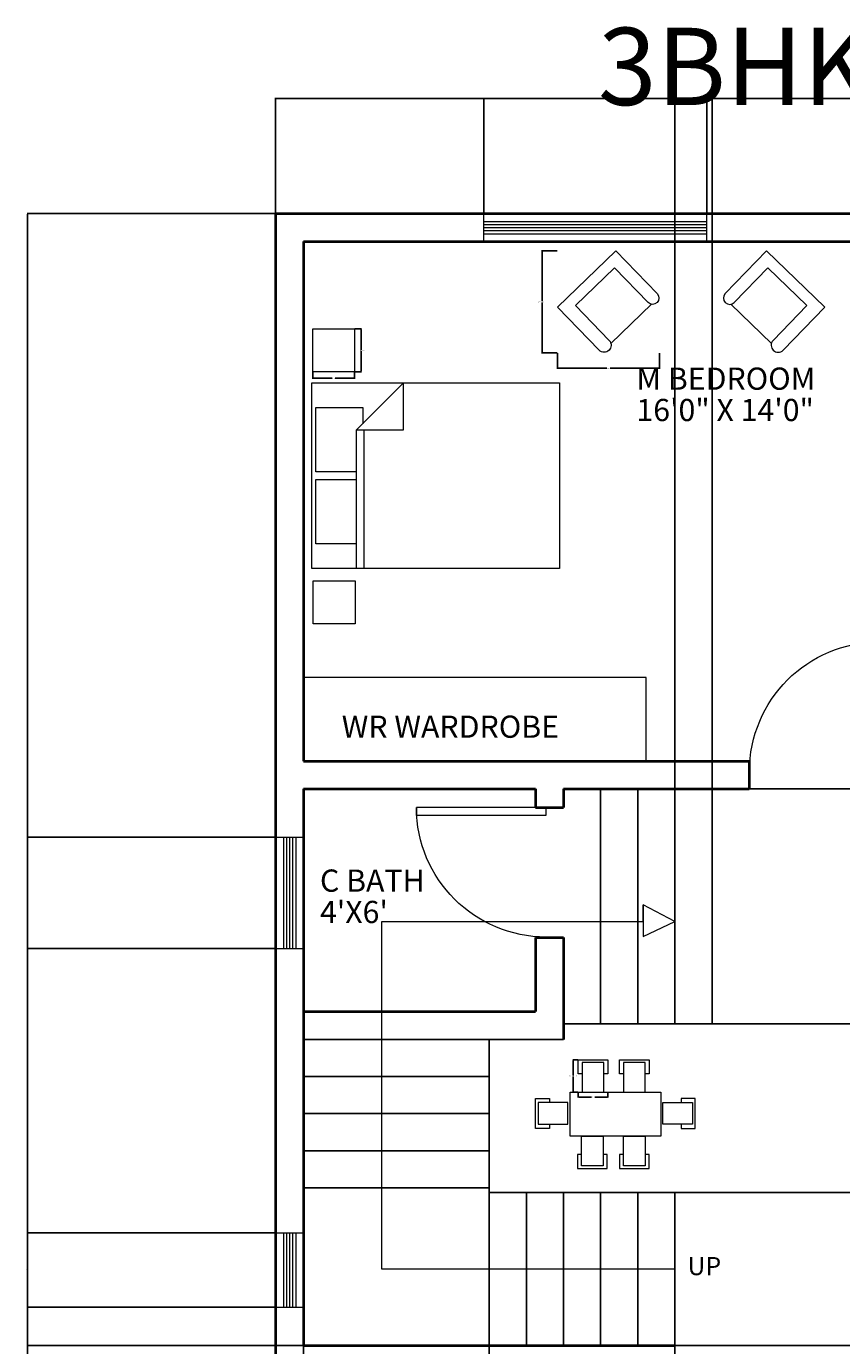
# Model space of a CAD drawing. Units: inches. Extents: x 12978 to 13669, y 46550 to 47327.
# Tile 3 of 5: x 12978 to 13242, y 46901 to 47327. Entities that reach past the tile are written whole.
import ezdxf

# ---------------------------------------------------------------- set-up
doc = ezdxf.new("R2010")
doc.units = ezdxf.units.IN
for name, color, linetype, lineweight in [('A-ANNO-DIMS', 2, 'Continuous', 18), ('A-ANNO-SYMB', 7, 'Continuous', 18), ('A-ANNO-TITL', 7, 'Continuous', 35), ('A-AREA-IDEN', 1, 'Continuous', 18), ('A-FLOR-CASE', 8, 'Continuous', 20), ('door', 4, 'Continuous', 20), ('furniture', 5, 'Continuous', 18), ('staircase', 7, 'Continuous', 25), ('text', 1, 'Continuous', 18), ('wall', 7, 'Continuous', 40), ('window', 1, 'Continuous', 18)]:
    doc.layers.add(name, color=color, linetype=linetype, lineweight=lineweight)
doc.styles.get("Standard").update_dxf_attribs({"font": 'arial.ttf'})
doc.dimstyles.get("Standard").update_dxf_attribs({"dimtxt": 0.18, "dimasz": 0.18, "dimexe": 0.18, "dimexo": 0.0625, "dimgap": 0.09, "dimtad": 0, "dimtih": 1, "dimtoh": 1, "dimdec": 4, "dimzin": 0, "dimdsep": 46, "dimtxsty": 'Standard', "dimcen": 0.09, "dimadec": 0, "dimazin": 0, "dimtfac": 1, "dimtdec": 4, "dimtofl": 0, "dimtmove": 0, "dimatfit": 3, "dimfxl": 1, "dimtolj": 1, "dimtzin": 0, "dimarcsym": 0})

# ---------------------------------------------------------------- blocks, each defined once
blk = doc.blocks.new('*U2')
for p, q in [((0, 0), (0, -100)), ((750, 0), (750, -100))]:
    blk.add_line(p, q)
blk.add_lwpolyline([(0, 0), (0, 750), (43.75, 750), (43.75, 0)], close=True)
blk.add_arc((0, 0), 750, 0, 90)
blk = doc.blocks.new('Bed - Queen')
for p, q in [((0, -80.00003), (0, 0)), ((0, 0), (59.99999, 0)), ((59.99999, 0), (59.99999, -80.00003)), ((7.99999, -1.2), (28.79998, -1.2)), ((7.99999, -14.4), (7.99999, -1.2)), ((28.79998, -1.2), (28.79998, -14.4)), ((31.19999, -1.2), (51.99999, -1.2)), ((31.19999, -14.4), (31.19999, -1.2)), ((51.99999, -1.2), (51.99999, -16.4)), ((0, -14.4), (44.8, -14.4)), ((44.8, -16.8), (0, -16.8)), ((59.99999, -29.6), (44.8, -14.4)), ((44.8, -14.4), (44.8, -29.6)), ((51.99999, -16.4), (46.79936, -16.4)), ((44.8, -29.6), (59.99999, -29.6)), ((59.99999, -80.00003), (0, -80.00003))]:
    blk.add_line(p, q)
blk = doc.blocks.new('WINDOW-72')
for p, q in [((0, 0), (0, 9)), ((72, 0), (72, 9)), ((0, 6.5), (72, 6.5)), ((0, 5.5), (72, 5.5)), ((0, 4.5), (72, 4.5)), ((0, 3.5), (72, 3.5)), ((0, 2.5), (72, 2.5))]:
    blk.add_line(p, q)
blk = doc.blocks.new('CHAIR-DINING')
for p, q in [((0, 0), (0, 9.65)), ((0, 9.65), (4.58, 9.65)), ((4.58, 9.65), (4.58, 8.35)), ((4.58, 0), (0, 0)), ((4.58, 1.31), (4.58, 0))]:
    blk.add_line(p, q)
blk.add_lwpolyline([(10.47, 8.35), (0.86, 8.35), (0.86, 1.31), (10.47, 1.31)], close=True)
blk = doc.blocks.new('CHAIR-BEDROOM')
for p, q in [((13.97, 32.78), (0.58, 18.95)), ((32.77, 14.58), (13.97, 32.78)), ((3.53, 16.1), (14.36, 27.28)), ((14.36, 27.28), (26.97, 15.07)), ((15.51, 2.82), (2.41, 15.5)), ((26.97, 15.07), (16.08, 3.82)), ((19.31, 0.69), (32.77, 14.58))]:
    blk.add_line(p, q)
for centre, radius in [((2.05, 17.52), 2.05), ((17.7, 2.25), 2.25)]:
    blk.add_arc(centre, radius, 135.9243, 315.9243)
blk = doc.blocks.new('TABLE-BEDSIDE')
blk.add_lwpolyline([(0, 13.86), (13.51, 13.86), (13.51, 0), (0, 0)], close=True)
blk = doc.blocks.new('*D25')
at = {"layer": 'A-ANNO-DIMS', "color": 0, "lineweight": -2, "transparency": 16777216}
for p, q in [((13084.59, 47229.35), (13086.79, 47229.35)), ((13086.61, 47229.17), (13086.61, 47222.6)), ((13086.61, 47215.66), (13086.61, 47222.23)), ((13084.59, 47215.48), (13086.79, 47215.48))]:
    blk.add_line(p, q, dxfattribs=at)
at = {"layer": 'A-ANNO-DIMS', "color": 0, "transparency": 16777216}
for points in [[(13086.58, 47229.17), (13086.64, 47229.17), (13086.61, 47229.35)], [(13086.58, 47215.66), (13086.64, 47215.66), (13086.61, 47215.48)]]:
    blk.add_solid(points, dxfattribs=at)
at = {"layer": 'Defpoints', "color": 0, "transparency": 16777216}
for p in [(13084.53, 47229.35), (13086.61, 47229.35), (13084.53, 47215.48)]:
    blk.add_point(p, dxfattribs=at)
at = {"layer": 'A-ANNO-DIMS', "color": 0, "transparency": 16777216, "insert": (13086.61, 47222.42), "char_height": 0.18, "attachment_point": 5}
blk.add_mtext('\\A1;SIDE TABLE 14 TYP.', dxfattribs=at)
blk = doc.blocks.new('*D26')
at = {"layer": 'A-ANNO-DIMS', "color": 0, "lineweight": -2, "transparency": 16777216}
for p, q in [((13071.02, 47215.42), (13071.02, 47213.22)), ((13071.2, 47213.4), (13077.25, 47213.4)), ((13084.35, 47213.4), (13078.29, 47213.4)), ((13084.53, 47215.42), (13084.53, 47213.22))]:
    blk.add_line(p, q, dxfattribs=at)
at = {"layer": 'A-ANNO-DIMS', "color": 0, "transparency": 16777216}
for points in [[(13071.2, 47213.43), (13071.2, 47213.37), (13071.02, 47213.4)], [(13084.35, 47213.43), (13084.35, 47213.37), (13084.53, 47213.4)]]:
    blk.add_solid(points, dxfattribs=at)
at = {"layer": 'Defpoints', "color": 0, "transparency": 16777216}
for p in [(13071.02, 47215.48), (13084.53, 47215.48), (13084.53, 47213.4)]:
    blk.add_point(p, dxfattribs=at)
at = {"layer": 'A-ANNO-DIMS', "color": 0, "transparency": 16777216, "insert": (13077.77, 47213.4), "char_height": 0.18, "attachment_point": 5}
blk.add_mtext('\\A1;14 TYP.', dxfattribs=at)
blk = doc.blocks.new('*D27')
at = {"layer": 'A-ANNO-DIMS', "color": 0, "lineweight": -2, "transparency": 16777216}
for p, q in [((13150.01, 47254.59), (13144.94, 47254.59)), ((13145.12, 47254.41), (13145.12, 47238.27)), ((13145.12, 47221.76), (13145.12, 47237.9)), ((13150.01, 47221.58), (13144.94, 47221.58))]:
    blk.add_line(p, q, dxfattribs=at)
at = {"layer": 'A-ANNO-DIMS', "color": 0, "transparency": 16777216}
for points in [[(13145.09, 47254.41), (13145.15, 47254.41), (13145.12, 47254.59)], [(13145.09, 47221.76), (13145.15, 47221.76), (13145.12, 47221.58)]]:
    blk.add_solid(points, dxfattribs=at)
at = {"layer": 'Defpoints', "color": 0, "transparency": 16777216}
for p in [(13145.12, 47254.59), (13150.07, 47254.59), (13150.07, 47221.58)]:
    blk.add_point(p, dxfattribs=at)
at = {"layer": 'A-ANNO-DIMS', "color": 0, "transparency": 16777216, "insert": (13145.12, 47238.09), "char_height": 0.18, "attachment_point": 5}
blk.add_mtext('\\A1;BEDROOM CHAIR 33 TYP.', dxfattribs=at)
blk = doc.blocks.new('*D28')
at = {"layer": 'A-ANNO-DIMS', "color": 0, "lineweight": -2, "transparency": 16777216}
for p, q in [((13150.07, 47221.51), (13150.07, 47216.45)), ((13183.05, 47221.51), (13183.05, 47216.45)), ((13150.25, 47216.63), (13166.04, 47216.63)), ((13182.87, 47216.63), (13167.09, 47216.63))]:
    blk.add_line(p, q, dxfattribs=at)
at = {"layer": 'A-ANNO-DIMS', "color": 0, "transparency": 16777216}
for points in [[(13150.25, 47216.66), (13150.25, 47216.6), (13150.07, 47216.63)], [(13182.87, 47216.66), (13182.87, 47216.6), (13183.05, 47216.63)]]:
    blk.add_solid(points, dxfattribs=at)
at = {"layer": 'Defpoints', "color": 0, "transparency": 16777216}
for p in [(13150.07, 47221.58), (13183.05, 47221.58), (13150.07, 47216.63)]:
    blk.add_point(p, dxfattribs=at)
at = {"layer": 'A-ANNO-DIMS', "color": 0, "transparency": 16777216, "insert": (13166.56, 47216.63), "char_height": 0.18, "attachment_point": 5}
blk.add_mtext('\\A1;33 TYP.', dxfattribs=at)
blk = doc.blocks.new('*D39')
at = {"layer": 'A-ANNO-DIMS', "color": 0, "lineweight": -2, "transparency": 16777216}
for p, q in [((13156.67, 46993.05), (13154.98, 46993.05)), ((13155.16, 46992.87), (13155.16, 46988)), ((13155.16, 46982.76), (13155.16, 46987.64)), ((13156.67, 46982.58), (13154.98, 46982.58))]:
    blk.add_line(p, q, dxfattribs=at)
at = {"layer": 'A-ANNO-DIMS', "color": 0, "transparency": 16777216}
for points in [[(13155.13, 46992.87), (13155.19, 46992.87), (13155.16, 46993.05)], [(13155.13, 46982.76), (13155.19, 46982.76), (13155.16, 46982.58)]]:
    blk.add_solid(points, dxfattribs=at)
at = {"layer": 'Defpoints', "color": 0, "transparency": 16777216}
for p in [(13156.73, 46993.05), (13155.16, 46982.58), (13156.73, 46982.58)]:
    blk.add_point(p, dxfattribs=at)
at = {"layer": 'A-ANNO-DIMS', "color": 0, "transparency": 16777216, "insert": (13155.16, 46987.82), "char_height": 0.18, "attachment_point": 5}
blk.add_mtext('\\A1;DINING CHAIR 10 TYP.', dxfattribs=at)
blk = doc.blocks.new('*D40')
at = {"layer": 'A-ANNO-DIMS', "color": 0, "lineweight": -2, "transparency": 16777216}
for p, q in [((13156.73, 46982.52), (13156.73, 46980.83)), ((13166.38, 46982.52), (13166.38, 46980.83)), ((13156.91, 46981.01), (13161.04, 46981.01)), ((13166.2, 46981.01), (13162.08, 46981.01))]:
    blk.add_line(p, q, dxfattribs=at)
at = {"layer": 'A-ANNO-DIMS', "color": 0, "transparency": 16777216}
for points in [[(13156.91, 46981.04), (13156.91, 46980.98), (13156.73, 46981.01)], [(13166.2, 46981.04), (13166.2, 46980.98), (13166.38, 46981.01)]]:
    blk.add_solid(points, dxfattribs=at)
at = {"layer": 'Defpoints', "color": 0, "transparency": 16777216}
for p in [(13156.73, 46982.58), (13166.38, 46982.58), (13166.38, 46981.01)]:
    blk.add_point(p, dxfattribs=at)
at = {"layer": 'A-ANNO-DIMS', "color": 0, "transparency": 16777216, "insert": (13161.56, 46981.01), "char_height": 0.18, "attachment_point": 5}
blk.add_mtext('\\A1;10 TYP.', dxfattribs=at)
blk = doc.blocks.new('*D51')
at = {"layer": 'A-ANNO-DIMS', "color": 0, "lineweight": -2, "transparency": 16777216}
for p, q in [((13059.01, 47266.7), (13059.01, 47304.06)), ((13059.19, 47303.88), (13321.22, 47303.88)), ((13583.83, 47303.88), (13321.79, 47303.88)), ((13584.01, 47266.7), (13584.01, 47304.06))]:
    blk.add_line(p, q, dxfattribs=at)
at = {"layer": 'A-ANNO-DIMS', "color": 0, "transparency": 16777216}
for points in [[(13059.19, 47303.91), (13059.19, 47303.85), (13059.01, 47303.88)], [(13583.83, 47303.91), (13583.83, 47303.85), (13584.01, 47303.88)]]:
    blk.add_solid(points, dxfattribs=at)
at = {"layer": 'Defpoints', "color": 0, "transparency": 16777216}
for p in [(13584.01, 47303.88), (13059.01, 47266.63), (13584.01, 47266.63)]:
    blk.add_point(p, dxfattribs=at)
at = {"layer": 'A-ANNO-DIMS', "color": 0, "transparency": 16777216, "insert": (13321.51, 47303.88), "char_height": 0.18, "attachment_point": 5}
blk.add_mtext('\\A1;525', dxfattribs=at)
blk = doc.blocks.new('*D52')
at = {"layer": 'A-ANNO-DIMS', "color": 0, "lineweight": -2, "transparency": 16777216}
for p, q in [((13058.94, 47266.63), (12978.69, 47266.63)), ((12978.87, 47266.45), (12978.87, 46963.82)), ((12978.87, 46660.81), (12978.87, 46963.45)), ((13058.94, 46660.63), (12978.69, 46660.63))]:
    blk.add_line(p, q, dxfattribs=at)
at = {"layer": 'A-ANNO-DIMS', "color": 0, "transparency": 16777216}
for points in [[(12978.84, 47266.45), (12978.9, 47266.45), (12978.87, 47266.63)], [(12978.84, 46660.81), (12978.9, 46660.81), (12978.87, 46660.63)]]:
    blk.add_solid(points, dxfattribs=at)
at = {"layer": 'Defpoints', "color": 0, "transparency": 16777216}
for p in [(12978.87, 47266.63), (13059.01, 47266.63), (13059.01, 46660.63)]:
    blk.add_point(p, dxfattribs=at)
at = {"layer": 'A-ANNO-DIMS', "color": 0, "transparency": 16777216, "insert": (12978.87, 46963.63), "char_height": 0.18, "attachment_point": 5}
blk.add_mtext('\\A1;606', dxfattribs=at)
blk = doc.blocks.new('*D53')
at = {"layer": 'A-ANNO-DIMS', "color": 0, "lineweight": -2, "transparency": 16777216}
for p, q in [((13059.01, 47266.7), (13059.01, 47304.06)), ((13059.19, 47303.88), (13092.27, 47303.88)), ((13126.14, 47303.88), (13093.06, 47303.88)), ((13126.32, 47266.7), (13126.32, 47304.06))]:
    blk.add_line(p, q, dxfattribs=at)
at = {"layer": 'A-ANNO-DIMS', "color": 0, "transparency": 16777216}
for points in [[(13059.19, 47303.91), (13059.19, 47303.85), (13059.01, 47303.88)], [(13126.14, 47303.91), (13126.14, 47303.85), (13126.32, 47303.88)]]:
    blk.add_solid(points, dxfattribs=at)
at = {"layer": 'Defpoints', "color": 0, "transparency": 16777216}
for p in [(13126.32, 47303.88), (13059.01, 47266.63), (13126.32, 47266.63)]:
    blk.add_point(p, dxfattribs=at)
at = {"layer": 'A-ANNO-DIMS', "color": 0, "transparency": 16777216, "insert": (13092.66, 47303.88), "char_height": 0.18, "attachment_point": 5}
blk.add_mtext('\\A1;67.32', dxfattribs=at)
blk = doc.blocks.new('*D54')
at = {"layer": 'A-ANNO-DIMS', "color": 0, "lineweight": -2, "transparency": 16777216}
for p, q in [((13198.32, 47266.7), (13198.32, 47304.06)), ((13198.5, 47303.88), (13242.72, 47303.88)), ((13287.73, 47303.88), (13243.51, 47303.88)), ((13287.91, 47266.7), (13287.91, 47304.06))]:
    blk.add_line(p, q, dxfattribs=at)
at = {"layer": 'A-ANNO-DIMS', "color": 0, "transparency": 16777216}
for points in [[(13198.5, 47303.91), (13198.5, 47303.85), (13198.32, 47303.88)], [(13287.73, 47303.91), (13287.73, 47303.85), (13287.91, 47303.88)]]:
    blk.add_solid(points, dxfattribs=at)
at = {"layer": 'Defpoints', "color": 0, "transparency": 16777216}
for p in [(13287.91, 47303.88), (13198.32, 47266.63), (13287.91, 47266.63)]:
    blk.add_point(p, dxfattribs=at)
at = {"layer": 'A-ANNO-DIMS', "color": 0, "transparency": 16777216, "insert": (13243.12, 47303.88), "char_height": 0.18, "attachment_point": 5}
blk.add_mtext('\\A1;89.59', dxfattribs=at)
blk = doc.blocks.new('*D66')
at = {"layer": 'A-ANNO-DIMS', "color": 0, "lineweight": -2, "transparency": 16777216}
for p, q in [((13058.94, 46913.08), (12978.69, 46913.08)), ((12978.87, 46912.9), (12978.87, 46907.04)), ((12978.87, 46900.81), (12978.87, 46906.68)), ((13067.94, 46900.63), (12978.69, 46900.63))]:
    blk.add_line(p, q, dxfattribs=at)
at = {"layer": 'A-ANNO-DIMS', "color": 0, "transparency": 16777216}
for points in [[(12978.84, 46912.9), (12978.9, 46912.9), (12978.87, 46913.08)], [(12978.84, 46900.81), (12978.9, 46900.81), (12978.87, 46900.63)]]:
    blk.add_solid(points, dxfattribs=at)
at = {"layer": 'Defpoints', "color": 0, "transparency": 16777216}
for p in [(12978.87, 46913.08), (13059.01, 46913.08), (13068.01, 46900.63)]:
    blk.add_point(p, dxfattribs=at)
at = {"layer": 'A-ANNO-DIMS', "color": 0, "transparency": 16777216, "insert": (12978.87, 46906.86), "char_height": 0.18, "attachment_point": 5}
blk.add_mtext('\\A1;12.448', dxfattribs=at)
blk = doc.blocks.new('*D67')
at = {"layer": 'A-ANNO-DIMS', "color": 0, "lineweight": -2, "transparency": 16777216}
for p, q in [((13058.94, 46937.07), (12978.69, 46937.07)), ((12978.87, 46936.89), (12978.87, 46925.26)), ((12978.87, 46913.26), (12978.87, 46924.89)), ((13058.94, 46913.08), (12978.69, 46913.08))]:
    blk.add_line(p, q, dxfattribs=at)
at = {"layer": 'A-ANNO-DIMS', "color": 0, "transparency": 16777216}
for points in [[(12978.84, 46936.89), (12978.9, 46936.89), (12978.87, 46937.07)], [(12978.84, 46913.26), (12978.9, 46913.26), (12978.87, 46913.08)]]:
    blk.add_solid(points, dxfattribs=at)
at = {"layer": 'Defpoints', "color": 0, "transparency": 16777216}
for p in [(12978.87, 46937.07), (13059.01, 46937.07), (13059.01, 46913.08)]:
    blk.add_point(p, dxfattribs=at)
at = {"layer": 'A-ANNO-DIMS', "color": 0, "transparency": 16777216, "insert": (12978.87, 46925.07), "char_height": 0.18, "attachment_point": 5}
blk.add_mtext('\\A1;23.984', dxfattribs=at)
blk = doc.blocks.new('*D68')
at = {"layer": 'A-ANNO-DIMS', "color": 0, "lineweight": -2, "transparency": 16777216}
for p, q in [((13058.94, 47029.05), (12978.69, 47029.05)), ((12978.87, 47028.87), (12978.87, 46983.24)), ((12978.87, 46937.25), (12978.87, 46982.88)), ((13058.94, 46937.07), (12978.69, 46937.07))]:
    blk.add_line(p, q, dxfattribs=at)
at = {"layer": 'A-ANNO-DIMS', "color": 0, "transparency": 16777216}
for points in [[(12978.84, 47028.87), (12978.9, 47028.87), (12978.87, 47029.05)], [(12978.84, 46937.25), (12978.9, 46937.25), (12978.87, 46937.07)]]:
    blk.add_solid(points, dxfattribs=at)
at = {"layer": 'Defpoints', "color": 0, "transparency": 16777216}
for p in [(12978.87, 47029.05), (13059.01, 47029.05), (13059.01, 46937.07)]:
    blk.add_point(p, dxfattribs=at)
at = {"layer": 'A-ANNO-DIMS', "color": 0, "transparency": 16777216, "insert": (12978.87, 46983.06), "char_height": 0.18, "attachment_point": 5}
blk.add_mtext('\\A1;91.99', dxfattribs=at)
blk = doc.blocks.new('*D69')
at = {"layer": 'A-ANNO-DIMS', "color": 0, "lineweight": -2, "transparency": 16777216}
for p, q in [((13058.94, 47065.05), (12978.69, 47065.05)), ((12978.87, 47064.87), (12978.87, 47047.24)), ((12978.87, 47029.23), (12978.87, 47046.87)), ((13058.94, 47029.05), (12978.69, 47029.05))]:
    blk.add_line(p, q, dxfattribs=at)
at = {"layer": 'A-ANNO-DIMS', "color": 0, "transparency": 16777216}
for points in [[(12978.84, 47064.87), (12978.9, 47064.87), (12978.87, 47065.05)], [(12978.84, 47029.23), (12978.9, 47029.23), (12978.87, 47029.05)]]:
    blk.add_solid(points, dxfattribs=at)
at = {"layer": 'Defpoints', "color": 0, "transparency": 16777216}
for p in [(12978.87, 47065.05), (13059.01, 47065.05), (13059.01, 47029.05)]:
    blk.add_point(p, dxfattribs=at)
at = {"layer": 'A-ANNO-DIMS', "color": 0, "transparency": 16777216, "insert": (12978.87, 47047.05), "char_height": 0.18, "attachment_point": 5}
blk.add_mtext('\\A1;36', dxfattribs=at)
blk = doc.blocks.new('*D70')
at = {"layer": 'A-ANNO-DIMS', "color": 0, "lineweight": -2, "transparency": 16777216}
for p, q in [((13128.01, 46951.57), (13128.01, 46549.88)), ((13068.01, 46900.57), (13068.01, 46549.88)), ((13068.19, 46550.06), (13097.79, 46550.06)), ((13127.83, 46550.06), (13098.22, 46550.06))]:
    blk.add_line(p, q, dxfattribs=at)
at = {"layer": 'A-ANNO-DIMS', "color": 0, "transparency": 16777216}
for points in [[(13068.19, 46550.09), (13068.19, 46550.03), (13068.01, 46550.06)], [(13127.83, 46550.09), (13127.83, 46550.03), (13128.01, 46550.06)]]:
    blk.add_solid(points, dxfattribs=at)
at = {"layer": 'Defpoints', "color": 0, "transparency": 16777216}
for p in [(13128.01, 46951.63), (13068.01, 46900.63), (13128.01, 46550.06)]:
    blk.add_point(p, dxfattribs=at)
at = {"layer": 'A-ANNO-DIMS', "color": 0, "transparency": 16777216, "insert": (13098.01, 46550.06), "char_height": 0.18, "attachment_point": 5}
blk.add_mtext('\\A1;60', dxfattribs=at)
blk = doc.blocks.new('*D71')
at = {"layer": 'A-ANNO-DIMS', "color": 0, "lineweight": -2, "transparency": 16777216}
for p, q in [((13128.01, 46950.07), (13128.01, 46549.88)), ((13188.01, 46900.57), (13188.01, 46549.88)), ((13128.19, 46550.06), (13157.79, 46550.06)), ((13187.83, 46550.06), (13158.22, 46550.06))]:
    blk.add_line(p, q, dxfattribs=at)
at = {"layer": 'A-ANNO-DIMS', "color": 0, "transparency": 16777216}
for points in [[(13128.19, 46550.09), (13128.19, 46550.03), (13128.01, 46550.06)], [(13187.83, 46550.09), (13187.83, 46550.03), (13188.01, 46550.06)]]:
    blk.add_solid(points, dxfattribs=at)
at = {"layer": 'Defpoints', "color": 0, "transparency": 16777216}
for p in [(13128.01, 46950.13), (13188.01, 46900.63), (13188.01, 46550.06)]:
    blk.add_point(p, dxfattribs=at)
at = {"layer": 'A-ANNO-DIMS', "color": 0, "transparency": 16777216, "insert": (13158.01, 46550.06), "char_height": 0.18, "attachment_point": 5}
blk.add_mtext('\\A1;60', dxfattribs=at)
blk = doc.blocks.new('*D72')
at = {"layer": 'A-ANNO-DIMS', "color": 0, "lineweight": -2, "transparency": 16777216}
for p, q in [((13188.07, 46950.13), (13669.26, 46950.13)), ((13669.08, 46949.95), (13669.08, 46925.57)), ((13669.08, 46900.81), (13669.08, 46925.2)), ((13188.07, 46900.63), (13669.26, 46900.63))]:
    blk.add_line(p, q, dxfattribs=at)
at = {"layer": 'A-ANNO-DIMS', "color": 0, "transparency": 16777216}
for points in [[(13669.05, 46949.95), (13669.11, 46949.95), (13669.08, 46950.13)], [(13669.05, 46900.81), (13669.11, 46900.81), (13669.08, 46900.63)]]:
    blk.add_solid(points, dxfattribs=at)
at = {"layer": 'Defpoints', "color": 0, "transparency": 16777216}
for p in [(13188.01, 46950.13), (13669.08, 46950.13), (13188.01, 46900.63)]:
    blk.add_point(p, dxfattribs=at)
at = {"layer": 'A-ANNO-DIMS', "color": 0, "transparency": 16777216, "insert": (13669.08, 46925.38), "char_height": 0.18, "attachment_point": 5}
blk.add_mtext('\\A1;49.5', dxfattribs=at)
blk = doc.blocks.new('*D73')
at = {"layer": 'A-ANNO-DIMS', "color": 0, "lineweight": -2, "transparency": 16777216}
for p, q in [((13200.07, 47080.63), (13669.26, 47080.63)), ((13669.08, 47080.45), (13669.08, 47042.85)), ((13669.08, 47004.87), (13669.08, 47042.48)), ((13200.07, 47004.69), (13669.26, 47004.69))]:
    blk.add_line(p, q, dxfattribs=at)
at = {"layer": 'A-ANNO-DIMS', "color": 0, "transparency": 16777216}
for points in [[(13669.05, 47080.45), (13669.11, 47080.45), (13669.08, 47080.63)], [(13669.05, 47004.87), (13669.11, 47004.87), (13669.08, 47004.69)]]:
    blk.add_solid(points, dxfattribs=at)
at = {"layer": 'Defpoints', "color": 0, "transparency": 16777216}
for p in [(13200.01, 47080.63), (13669.08, 47080.63), (13200.01, 47004.69)]:
    blk.add_point(p, dxfattribs=at)
at = {"layer": 'A-ANNO-DIMS', "color": 0, "transparency": 16777216, "insert": (13669.08, 47042.66), "char_height": 0.18, "attachment_point": 5}
blk.add_mtext('\\A1;75.94', dxfattribs=at)
blk = doc.blocks.new('*D74')
at = {"layer": 'A-ANNO-DIMS', "color": 0, "lineweight": -2, "transparency": 16777216}
for p, q in [((13188.01, 47080.7), (13188.01, 47304.06)), ((13188.19, 47303.88), (13193.8, 47303.88)), ((13199.83, 47303.88), (13194.21, 47303.88)), ((13200.01, 47080.7), (13200.01, 47304.06))]:
    blk.add_line(p, q, dxfattribs=at)
at = {"layer": 'A-ANNO-DIMS', "color": 0, "transparency": 16777216}
for points in [[(13188.19, 47303.91), (13188.19, 47303.85), (13188.01, 47303.88)], [(13199.83, 47303.91), (13199.83, 47303.85), (13200.01, 47303.88)]]:
    blk.add_solid(points, dxfattribs=at)
at = {"layer": 'Defpoints', "color": 0, "transparency": 16777216}
for p in [(13200.01, 47303.88), (13188.01, 47080.63), (13200.01, 47080.63)]:
    blk.add_point(p, dxfattribs=at)
at = {"layer": 'A-ANNO-DIMS', "color": 0, "transparency": 16777216, "insert": (13194.01, 47303.88), "char_height": 0.18, "attachment_point": 5}
blk.add_mtext('\\A1;12', dxfattribs=at)

msp = doc.modelspace()

# ---------------------------------------------------------------- linework, layer by layer
at = {"layer": 'A-ANNO-SYMB'}
for p, q in [((13177.713, 47037.7812), (13177.713, 47043.1818)), ((13177.713, 47043.1818), (13177.713, 47032.9062)), ((13188.005, 47037.804), (13177.713, 47043.1818)), ((13093.2989, 46925.3845), (13093.2989, 47037.7812)), ((13093.2989, 47037.7812), (13177.713, 47037.7812)), ((13177.713, 47032.9062), (13188.005, 47037.804)), ((13188.005, 46925.3845), (13093.2989, 46925.3845))]:
    msp.add_line(p, q, dxfattribs=at)
at = {"layer": 'A-FLOR-CASE'}
msp.add_lwpolyline([(13068.005, 47089.6345), (13178.7109, 47089.6345), (13178.7109, 47116.6058), (13068.005, 47116.6058)], close=True, dxfattribs=at)
at = {"layer": 'furniture'}
msp.add_lwpolyline([(13154.1121, 46982.5831), (13183.4086, 46982.5831), (13183.4086, 46968.3342), (13154.1121, 46968.3342)], close=True, dxfattribs=at)
at = {"layer": 'staircase'}
for p, q in [((13164.005, 47080.6345), (13164.005, 47004.6918)), ((13176.005, 47080.6345), (13176.005, 47004.6918)), ((13188.005, 47080.6345), (13188.005, 47004.6918)), ((13200.005, 47080.6345), (13200.005, 47004.6918)), ((13152.005, 47004.6918), (13200.005, 47004.6918)), ((13068.005, 46999.6345), (13152.005, 46999.6345)), ((13128.005, 46999.6345), (13128.005, 46900.6345)), ((13068.005, 46987.6345), (13128.005, 46987.6345)), ((13068.005, 46975.6345), (13128.005, 46975.6345)), ((13068.005, 46963.6345), (13128.005, 46963.6345)), ((13068.005, 46951.6345), (13128.005, 46951.6345)), ((13128.005, 46950.1345), (13188.005, 46950.1345)), ((13140.005, 46900.6345), (13140.005, 46950.1345)), ((13152.005, 46900.6345), (13152.005, 46950.1345)), ((13164.005, 46900.6345), (13164.005, 46950.1345)), ((13176.005, 46900.6345), (13176.005, 46950.1345)), ((13188.005, 46950.1345), (13188.005, 46900.6345)), ((13188.005, 46900.6345), (13188.005, 46950.1345))]:
    msp.add_line(p, q, dxfattribs=at)
at = {"layer": 'wall'}
for p, q in [((13059.005, 47266.6345), (13584.005, 47266.6345)), ((13059.005, 47266.6345), (13059.005, 46821.1345)), ((13068.005, 47257.6345), (13068.005, 47089.6345)), ((13068.005, 47257.6345), (13260.005, 47257.6345)), ((13068.005, 47089.6345), (13212.005, 47089.6345)), ((13212.005, 47089.6345), (13212.005, 47080.6345)), ((13068.005, 47080.6345), (13143.005, 47080.6345)), ((13068.005, 47080.6345), (13068.005, 46900.6345)), ((13143.005, 47080.6345), (13143.005, 47074.6345)), ((13152.005, 47080.6345), (13152.005, 47074.6345)), ((13152.005, 47080.6345), (13212.005, 47080.6345)), ((13143.005, 47074.6345), (13152.005, 47074.6345)), ((13143.005, 47032.6345), (13152.005, 47032.6345)), ((13143.005, 47032.6345), (13143.005, 47008.6345)), ((13152.005, 47032.6345), (13152.005, 46999.6345)), ((13068.005, 47008.6345), (13143.005, 47008.6345)), ((13068.005, 46900.6345), (13188.005, 46900.6345))]:
    msp.add_line(p, q, dxfattribs=at)
at = {"layer": 'window'}
for p, q in [((13059.005, 47065.0544), (13068.005, 47065.0544)), ((13061.505, 47065.0544), (13061.505, 47029.0544)), ((13062.505, 47065.0544), (13062.505, 47029.0544)), ((13063.505, 47065.0544), (13063.505, 47029.0544)), ((13064.505, 47065.0544), (13064.505, 47029.0544)), ((13065.505, 47065.0544), (13065.505, 47029.0544)), ((13059.005, 47029.0544), (13068.005, 47029.0544)), ((13059.005, 46937.0671), (13068.005, 46937.0671)), ((13061.505, 46937.0671), (13061.505, 46913.0827)), ((13062.505, 46937.0671), (13062.505, 46913.0827)), ((13063.505, 46937.0671), (13063.505, 46913.0827)), ((13064.505, 46937.0671), (13064.505, 46913.0827)), ((13065.505, 46937.0671), (13065.505, 46913.0827)), ((13059.005, 46913.0827), (13068.005, 46913.0827))]:
    msp.add_line(p, q, dxfattribs=at)

# ---------------------------------------------------------------- block references
at = {"layer": 'door', "xscale": -0.0558759688399716, "yscale": 0.0558759688399716, "zscale": 0.0558759688399716}
msp.add_blockref('*U2', (13254.005, 47086.222), dxfattribs=at)
at = {"layer": 'door', "xscale": -0.0558759688399716, "yscale": 0.0558759688399716, "zscale": 0.0558759688399716, "rotation": 90}
msp.add_blockref('*U2', (13146.4174, 47074.6345), dxfattribs=at)
at = {"layer": 'furniture', "extrusion": (0, 0, -1), "zscale": -1}
for name, p in [('CHAIR-BEDROOM', (-13182.8436, 47221.8087)), ('CHAIR-DINING', (-13194.5931, 46970.8799))]:
    msp.add_blockref(name, p, dxfattribs=at)
at = {"layer": 'furniture'}
for name, p in [('CHAIR-BEDROOM', (13203.6559, 47221.8087)), ('TABLE-BEDSIDE', (13071.0152, 47215.4832)), ('TABLE-BEDSIDE', (13071.1875, 47133.9989)), ('CHAIR-DINING', (13142.9276, 46970.8799))]:
    msp.add_blockref(name, p, dxfattribs=at)
for name, p, rotation in [('Bed - Queen', (13070.7494, 47151.9157), 90), ('CHAIR-DINING', (13156.7295, 46993.0546), 269.9999999999294), ('CHAIR-DINING', (13170.0547, 46993.0546), 269.9999999999294)]:
    msp.add_blockref(name, p, dxfattribs=dict(at, rotation=rotation))
at = {"layer": 'furniture', "extrusion": (0, 0, -1), "zscale": -1}
for p, rotation in [((-13156.4944, 46957.8627), 89.99999999997382), ((-13170.0547, 46957.8627), 89.99999999998592)]:
    msp.add_blockref('CHAIR-DINING', p, dxfattribs=dict(at, rotation=rotation))
at = {"layer": 'window'}
msp.add_blockref('WINDOW-72', (13126.3221, 47257.6345), dxfattribs=at)

# ---------------------------------------------------------------- texts
at = {"layer": 'A-ANNO-TITL'}
msp.add_text('3BHK HOUSE PLAN', height=25.000014, dxfattribs=at).set_placement((13163.1704, 47301.722))
at = {"layer": 'A-AREA-IDEN'}
for s, height, p in [('M BEDROOM', 7.17855, (13175.5707, 47209.6808)), ('16\'0" X 14\'0"', 7.178549, (13175.5707, 47199.5424)), ('C BATH', 7.17855, (13073.3397, 47047.3867)), ("4'X6'", 7.17855, (13073.3397, 47037.2483))]:
    msp.add_text(s, height=height, dxfattribs=at).set_placement(p)
at = {"layer": 'text'}
for s, height, p in [('WR WARDROBE', 7.178549, (13080.3602, 47097.1552)), ('UP', 5.89168, (13192.0558, 46923.4027))]:
    msp.add_text(s, height=height, dxfattribs=at).set_placement(p)

# ---------------------------------------------------------------- dimensions: what is measured, and where the dimension line sits
at = {"layer": 'A-ANNO-DIMS'}
for base, p1, p2, override, picture, middle in [((13584.005, 47303.8845), (13059.005, 47266.6345), (13584.005, 47266.6345), {"dimdec": 0, "dimlfac": 1, "dimrnd": 0, "dimzin": 0, "dimdsep": 46, "dimlunit": 2}, '*D51', (13321.505, 47303.8845)), ((13126.3221, 47303.8845), (13059.005, 47266.6345), (13126.3221, 47266.6345), {"dimdec": 2, "dimlfac": 1, "dimrnd": 0, "dimzin": 0, "dimdsep": 46, "dimlunit": 2}, '*D53', (13092.6636, 47303.8845)), ((13200.005, 47303.8845), (13188.005, 47080.6345), (13200.005, 47080.6345), {"dimdec": 0, "dimlfac": 1, "dimrnd": 0, "dimzin": 0, "dimdsep": 46, "dimlunit": 2}, '*D74', (13194.005, 47303.8845)), ((13287.9094, 47303.8845), (13198.3221, 47266.6345), (13287.9094, 47266.6345), {"dimdec": 2, "dimlfac": 1, "dimrnd": 0, "dimzin": 0, "dimdsep": 46, "dimlunit": 2}, '*D54', (13243.1158, 47303.8845)), ((13128.005, 46550.0575), (13068.005, 46900.6345), (13128.005, 46951.6345), {"dimdec": 0, "dimlfac": 1, "dimrnd": 0, "dimzin": 0, "dimdsep": 46, "dimlunit": 2}, '*D70', (13098.005, 46550.0575)), ((13188.005, 46550.0575), (13128.005, 46950.1345), (13188.005, 46900.6345), {"dimdec": 0, "dimlfac": 1, "dimrnd": 0, "dimzin": 0, "dimdsep": 46, "dimlunit": 2}, '*D71', (13158.005, 46550.0575))]:
    dim = msp.add_linear_dim(base=base, p1=p1, p2=p2, dimstyle='Standard', override=override, dxfattribs=at)
    dim.commit()
    dim.dimension.update_dxf_attribs({"geometry": picture, "text_midpoint": middle})
for base, p1, p2, override, picture, middle in [((12978.8702, 47266.6345), (13059.005, 46660.6345), (13059.005, 47266.6345), {"dimdec": 0, "dimlfac": 1, "dimrnd": 0, "dimzin": 0, "dimdsep": 46, "dimlunit": 2}, '*D52', (12978.8702, 46963.6345)), ((13669.0793, 47080.6345), (13200.005, 47004.6918), (13200.005, 47080.6345), {"dimdec": 2, "dimlfac": 1, "dimrnd": 0, "dimzin": 0, "dimdsep": 46, "dimlunit": 2}, '*D73', (13669.0793, 47042.6631)), ((12978.8702, 47065.0544), (13059.005, 47029.0544), (13059.005, 47065.0544), {"dimdec": 0, "dimlfac": 1, "dimrnd": 0, "dimzin": 0, "dimdsep": 46, "dimlunit": 2}, '*D69', (12978.8702, 47047.0544)), ((12978.8702, 47029.0544), (13059.005, 46937.0671), (13059.005, 47029.0544), {"dimdec": 2, "dimlfac": 1, "dimrnd": 0, "dimzin": 0, "dimdsep": 46, "dimlunit": 2}, '*D68', (12978.8702, 46983.0607)), ((13669.0793, 46950.1345), (13188.005, 46900.6345), (13188.005, 46950.1345), {"dimdec": 1, "dimlfac": 1, "dimrnd": 0, "dimzin": 0, "dimdsep": 46, "dimlunit": 2}, '*D72', (13669.0793, 46925.3845)), ((12978.8702, 46937.0671), (13059.005, 46913.0827), (13059.005, 46937.0671), {"dimdec": 3, "dimlfac": 1, "dimrnd": 0, "dimzin": 0, "dimdsep": 46, "dimlunit": 2}, '*D67', (12978.8702, 46925.0749)), ((12978.8702, 46913.0827), (13068.005, 46900.6345), (13059.005, 46913.0827), {"dimdec": 3, "dimlfac": 1, "dimrnd": 0, "dimzin": 0, "dimdsep": 46, "dimlunit": 2}, '*D66', (12978.8702, 46906.8586))]:
    dim = msp.add_linear_dim(base=base, p1=p1, p2=p2, angle=90, dimstyle='Standard', override=override, dxfattribs=at)
    dim.commit()
    dim.dimension.update_dxf_attribs({"geometry": picture, "text_midpoint": middle})
for base, p1, p2, angle, text, picture, middle in [((13145.1214, 47254.5927), (13150.0737, 47221.5775), (13150.0737, 47254.5927), 90, 'BEDROOM CHAIR <> TYP.', '*D27', (13145.1214, 47238.0851)), ((13086.6086, 47229.3469), (13084.529, 47215.4832), (13084.529, 47229.3469), 90, 'SIDE TABLE <> TYP.', '*D25', (13086.6086, 47222.4151)), ((13150.0737, 47216.6252), (13183.0543, 47221.5775), (13150.0737, 47221.5775), 180, '<> TYP.', '*D28', (13166.564, 47216.6252)), ((13155.1588, 46982.5831), (13156.7295, 46993.0546), (13156.7295, 46982.5831), 270, 'DINING CHAIR <> TYP.', '*D39', (13155.1588, 46987.8189))]:
    dim = msp.add_linear_dim(base=base, p1=p1, p2=p2, angle=angle, text=text, dimstyle='Standard', override={"dimdec": 0, "dimlfac": 1, "dimrnd": 0, "dimzin": 0, "dimdsep": 46, "dimlunit": 2}, dxfattribs=at)
    dim.commit()
    dim.dimension.update_dxf_attribs({"geometry": picture, "text_midpoint": middle})
for base, p1, p2, picture, middle in [((13084.529, 47213.4037), (13071.0152, 47215.4832), (13084.529, 47215.4832), '*D26', (13077.7721, 47213.4037)), ((13166.3823, 46981.0124), (13156.7295, 46982.5831), (13166.3823, 46982.5831), '*D40', (13161.5559, 46981.0124))]:
    dim = msp.add_linear_dim(base=base, p1=p1, p2=p2, text='<> TYP.', dimstyle='Standard', override={"dimdec": 0, "dimlfac": 1, "dimrnd": 0, "dimzin": 0, "dimdsep": 46, "dimlunit": 2}, dxfattribs=at)
    dim.commit()
    dim.dimension.update_dxf_attribs({"geometry": picture, "text_midpoint": middle})

doc.saveas('drawing.dxf')
